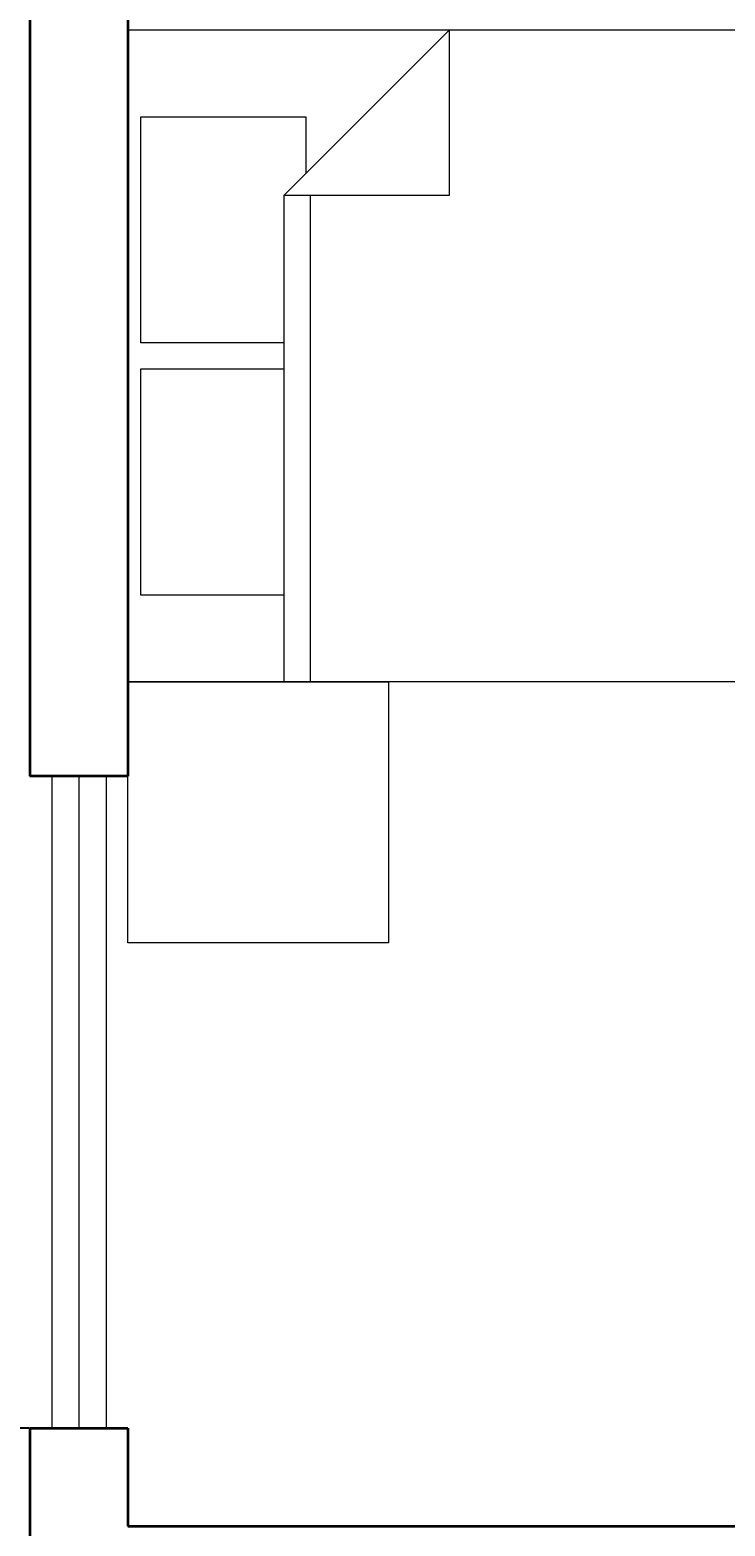
# Model space of a CAD drawing. Units: inches. Extents: x -4843 to -3402, y -164 to 3629.
# Tile 9 of 22: x -4596 to -4532, y 828 to 966. Entities that reach past the tile are written whole.
import ezdxf

# ---------------------------------------------------------------- set-up
doc = ezdxf.new("R2010")
doc.units = ezdxf.units.IN
for name, color, linetype, lineweight in [('A-ANNO-DIMS', 2, 'Continuous', 18), ('furniture', 6, 'Continuous', 18), ('walls', 7, 'Continuous', 35), ('windows', 1, 'Continuous', 18)]:
    doc.layers.add(name, color=color, linetype=linetype, lineweight=lineweight)
doc.styles.get("Standard").update_dxf_attribs({"font": 'arial.ttf'})
doc.dimstyles.get("Standard").update_dxf_attribs({"dimtxt": 0.18, "dimasz": 0.18, "dimexe": 0.18, "dimexo": 0.0625, "dimgap": 0.09, "dimtad": 0, "dimtih": 1, "dimtoh": 1, "dimdec": 4, "dimzin": 0, "dimdsep": 46, "dimtxsty": 'Standard', "dimcen": 0.09, "dimadec": 0, "dimazin": 0, "dimtfac": 1, "dimtdec": 4, "dimtofl": 0, "dimtmove": 0, "dimatfit": 3, "dimfxl": 1, "dimtolj": 1, "dimtzin": 0, "dimarcsym": 0})

# ---------------------------------------------------------------- blocks, each defined once
blk = doc.blocks.new('window')
at = {"layer": 'windows'}
for p, q in [((0, 7), (60, 7)), ((0, 4.5), (60, 4.5)), ((0, 2), (60, 2))]:
    blk.add_line(p, q, dxfattribs=at)
for points in [[(0, 9), (0, 0)], [(60, 0), (60, 9)]]:
    blk.add_lwpolyline(points, dxfattribs=at)
blk = doc.blocks.new('Bed - Queen')
for p, q in [((0, -80.00003), (0, 0)), ((0, 0), (59.99999, 0)), ((59.99999, 0), (59.99999, -80.00003)), ((7.99999, -1.2), (28.79998, -1.2)), ((7.99999, -14.4), (7.99999, -1.2)), ((28.79998, -1.2), (28.79998, -14.4)), ((31.19999, -1.2), (51.99999, -1.2)), ((31.19999, -14.4), (31.19999, -1.2)), ((51.99999, -1.2), (51.99999, -16.4)), ((0, -14.4), (44.8, -14.4)), ((59.99999, -29.6), (44.8, -14.4)), ((44.8, -14.4), (44.8, -29.6)), ((51.99999, -16.4), (46.79936, -16.4)), ((44.8, -16.8), (0, -16.8)), ((44.8, -29.6), (59.99999, -29.6)), ((59.99999, -80.00003), (0, -80.00003))]:
    blk.add_line(p, q)
blk = doc.blocks.new('NIGHTSTAND-24IN')
blk.add_lwpolyline([(0, 24), (24, 24), (24, 0), (0, 0)], close=True)
blk = doc.blocks.new('*D74')
at = {"layer": 'A-ANNO-DIMS', "color": 0, "lineweight": -2, "transparency": 16777216}
for p, q in [((-4595.85, 837.35), (-4842.55, 837.35)), ((-4842.37, 837.17), (-4842.37, 828.54)), ((-4842.37, 819.53), (-4842.37, 828.17)), ((-4586.85, 819.35), (-4842.55, 819.35))]:
    blk.add_line(p, q, dxfattribs=at)
at = {"layer": 'A-ANNO-DIMS', "color": 0, "transparency": 16777216}
for points in [[(-4842.4, 837.17), (-4842.34, 837.17), (-4842.37, 837.35)], [(-4842.4, 819.53), (-4842.34, 819.53), (-4842.37, 819.35)]]:
    blk.add_solid(points, dxfattribs=at)
at = {"layer": 'Defpoints', "color": 0, "transparency": 16777216}
for p in [(-4595.78, 837.35), (-4842.37, 819.35), (-4586.78, 819.35)]:
    blk.add_point(p, dxfattribs=at)
at = {"layer": 'A-ANNO-DIMS', "color": 0, "transparency": 16777216, "insert": (-4842.37, 828.35), "char_height": 0.18, "attachment_point": 5}
blk.add_mtext('\\A1;18', dxfattribs=at)

msp = doc.modelspace()

# ---------------------------------------------------------------- linework, layer by layer
at = {"layer": 'walls'}
for p, q in [((-4595.78, 1020.35), (-4595.78, 897.35)), ((-4586.78, 1011.35), (-4586.78, 897.35)), ((-4595.78, 837.35), (-4595.78, 793.85)), ((-4586.78, 837.35), (-4586.78, 828.35)), ((-4586.78, 828.35), (-4460.78, 828.35))]:
    msp.add_line(p, q, dxfattribs=at)
for points in [[(-4586.78, 897.35), (-4595.78, 897.35)], [(-4595.78, 837.35), (-4586.78, 837.35)]]:
    msp.add_lwpolyline(points, dxfattribs=at)

# ---------------------------------------------------------------- block references
at = {"layer": 'furniture'}
for name, p, rotation in [('Bed - Queen', (-4586.78, 906.02), 90), ('NIGHTSTAND-24IN', (-4562.78, 882.02), 89.99999999999774)]:
    msp.add_blockref(name, p, dxfattribs=dict(at, rotation=rotation))
at = {"layer": 'windows', "rotation": 270}
msp.add_blockref('window', (-4595.78, 897.35), dxfattribs=at)

# ---------------------------------------------------------------- dimensions: what is measured, and where the dimension line sits
at = {"layer": 'A-ANNO-DIMS'}
dim = msp.add_linear_dim(base=(-4842.37, 819.35), p1=(-4595.78, 837.35), p2=(-4586.78, 819.35), angle=90, dimstyle='Standard', override={"dimdec": 0, "dimlfac": 1, "dimrnd": 0, "dimzin": 0, "dimdsep": 46, "dimlunit": 2}, dxfattribs=at)
dim.commit()
dim.dimension.update_dxf_attribs({"geometry": '*D74', "text_midpoint": (-4842.37, 828.35)})

doc.saveas('drawing.dxf')
